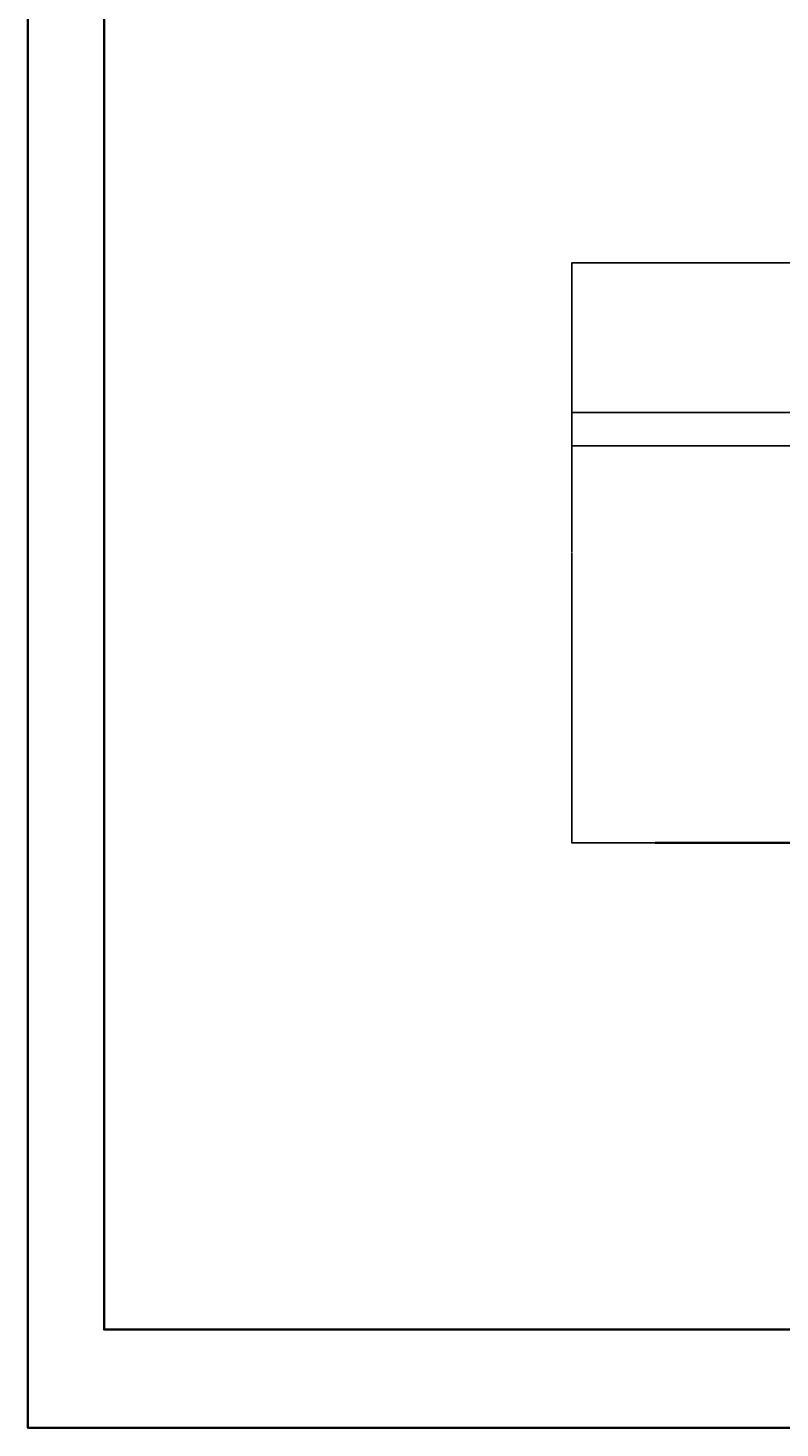
# Model space of a CAD drawing. Units: inches. Extents: x -934 to 898, y -1502 to 444.
# Tile 1 of 10: x -934 to -524, y -1502 to -739. Entities that reach past the tile are written whole.
import ezdxf

# ---------------------------------------------------------------- set-up
doc = ezdxf.new("R2010")
doc.units = ezdxf.units.IN
doc.header["$MEASUREMENT"] = 0
for name, color, linetype, lineweight in [('A-ANNO-DIMS', 2, 'Continuous', 18), ('A-ANNO-TTLB', 7, 'Continuous', 35), ('L-GRND', 7, 'Continuous', 35)]:
    doc.layers.add(name, color=color, linetype=linetype, lineweight=lineweight)
doc.styles.get("Standard").update_dxf_attribs({"font": 'arial.ttf'})
doc.dimstyles.get("Standard").update_dxf_attribs({"dimtxt": 0.18, "dimasz": 0.18, "dimexe": 0.18, "dimexo": 0.0625, "dimgap": 0.09, "dimtad": 0, "dimtih": 1, "dimtoh": 1, "dimdec": 4, "dimzin": 0, "dimdsep": 46, "dimtxsty": 'Standard', "dimcen": 0.09, "dimadec": 0, "dimazin": 0, "dimtfac": 1, "dimtdec": 4, "dimtofl": 0, "dimtmove": 0, "dimatfit": 3, "dimfxl": 1, "dimtolj": 1, "dimtzin": 0, "dimarcsym": 0})

# ---------------------------------------------------------------- blocks, each defined once
blk = doc.blocks.new('*D114')
at = {"layer": 'A-ANNO-DIMS', "color": 0, "lineweight": -2, "transparency": 16777216}
for p, q in [((-122.37, -948.66), (-637.55, -948.66)), ((-637.37, -948.84), (-637.37, -957.63)), ((-637.37, -966.78), (-637.37, -957.99)), ((-142.26, -966.96), (-637.55, -966.96))]:
    blk.add_line(p, q, dxfattribs=at)
at = {"layer": 'A-ANNO-DIMS', "color": 0, "transparency": 16777216}
for points in [[(-637.4, -948.84), (-637.34, -948.84), (-637.37, -948.66)], [(-637.4, -966.78), (-637.34, -966.78), (-637.37, -966.96)]]:
    blk.add_solid(points, dxfattribs=at)
at = {"layer": 'Defpoints', "color": 0, "transparency": 16777216}
for p in [(-637.37, -948.66), (-122.31, -948.66), (-142.19, -966.96)]:
    blk.add_point(p, dxfattribs=at)
at = {"layer": 'A-ANNO-DIMS', "color": 0, "transparency": 16777216, "insert": (-637.37, -957.81), "char_height": 0.18, "attachment_point": 5}
blk.add_mtext('\\A1;18.294', dxfattribs=at)
blk = doc.blocks.new('*D117')
at = {"layer": 'A-ANNO-DIMS', "color": 0, "lineweight": -2, "transparency": 16777216}
for p, q in [((-490.58, -867.34), (-637.55, -867.34)), ((-637.37, -867.52), (-637.37, -1024.99)), ((-637.37, -1182.83), (-637.37, -1025.36)), ((-448.1, -1183.01), (-637.55, -1183.01))]:
    blk.add_line(p, q, dxfattribs=at)
at = {"layer": 'A-ANNO-DIMS', "color": 0, "transparency": 16777216}
for points in [[(-637.4, -867.52), (-637.34, -867.52), (-637.37, -867.34)], [(-637.4, -1182.83), (-637.34, -1182.83), (-637.37, -1183.01)]]:
    blk.add_solid(points, dxfattribs=at)
at = {"layer": 'Defpoints', "color": 0, "transparency": 16777216}
for p in [(-637.37, -867.34), (-490.52, -867.34), (-448.04, -1183.01)]:
    blk.add_point(p, dxfattribs=at)
at = {"layer": 'A-ANNO-DIMS', "color": 0, "transparency": 16777216, "insert": (-637.37, -1025.17), "char_height": 0.18, "attachment_point": 5}
blk.add_mtext('\\A1;315.7', dxfattribs=at)

msp = doc.modelspace()

# ---------------------------------------------------------------- linework, layer by layer
at = {"layer": 'A-ANNO-TTLB'}
for points in [[(-933.5092, 444.4646), (897.7239, 444.4646), (897.7239, -1501.5858), (-933.5092, -1501.5858)], [(-892.081, 380.0228), (832.9871, 380.0228), (832.9871, -1448.0237), (-892.081, -1448.0237)]]:
    msp.add_lwpolyline(points, close=True, dxfattribs=at)
at = {"layer": 'L-GRND'}
msp.add_line((-288.9776, -1183.0104), (-591.8658, -1183.0104), dxfattribs=at)

# ---------------------------------------------------------------- dimensions: what is measured, and where the dimension line sits
at = {"layer": 'A-ANNO-DIMS'}
for base, p1, p2, override, picture, middle in [((-637.3658, -867.3393), (-448.0415, -1183.0104), (-490.5224, -867.3393), {"dimdec": 1, "dimlfac": 1, "dimrnd": 0, "dimzin": 0, "dimdsep": 46, "dimlunit": 2}, '*D117', (-637.3658, -1025.1749)), ((-637.3658, -948.6643), (-142.1926, -966.9581), (-122.305, -948.6643), {"dimdec": 3, "dimlfac": 1, "dimrnd": 0, "dimzin": 0, "dimdsep": 46, "dimlunit": 2}, '*D114', (-637.3658, -957.8112))]:
    dim = msp.add_linear_dim(base=base, p1=p1, p2=p2, angle=90, dimstyle='Standard', override=override, dxfattribs=at)
    dim.commit()
    dim.dimension.update_dxf_attribs({"geometry": picture, "text_midpoint": middle})

doc.saveas('drawing.dxf')
